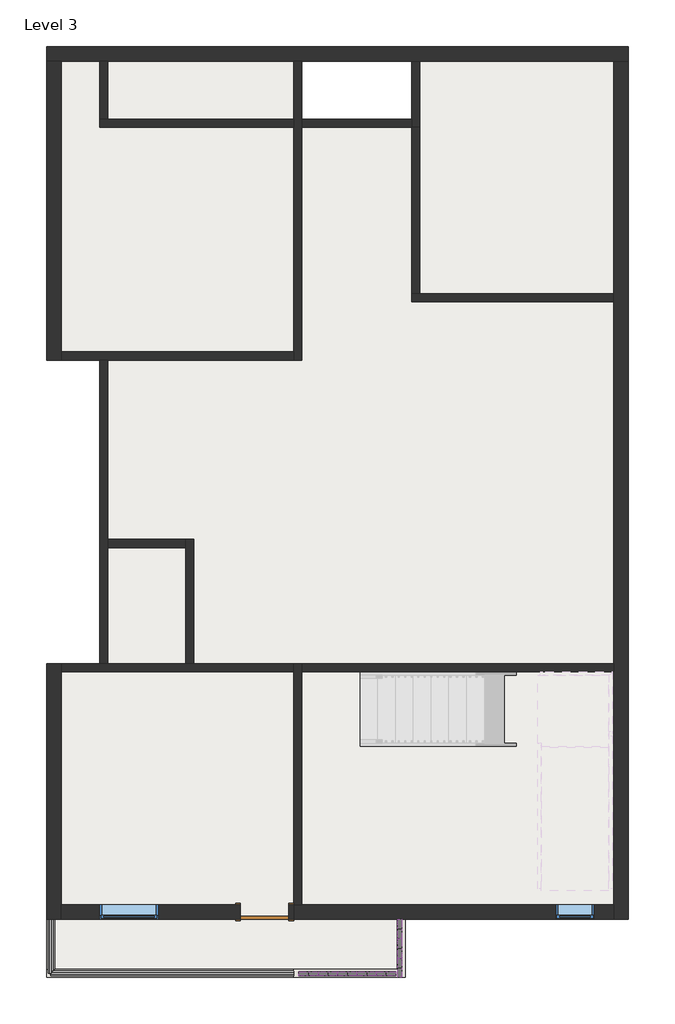
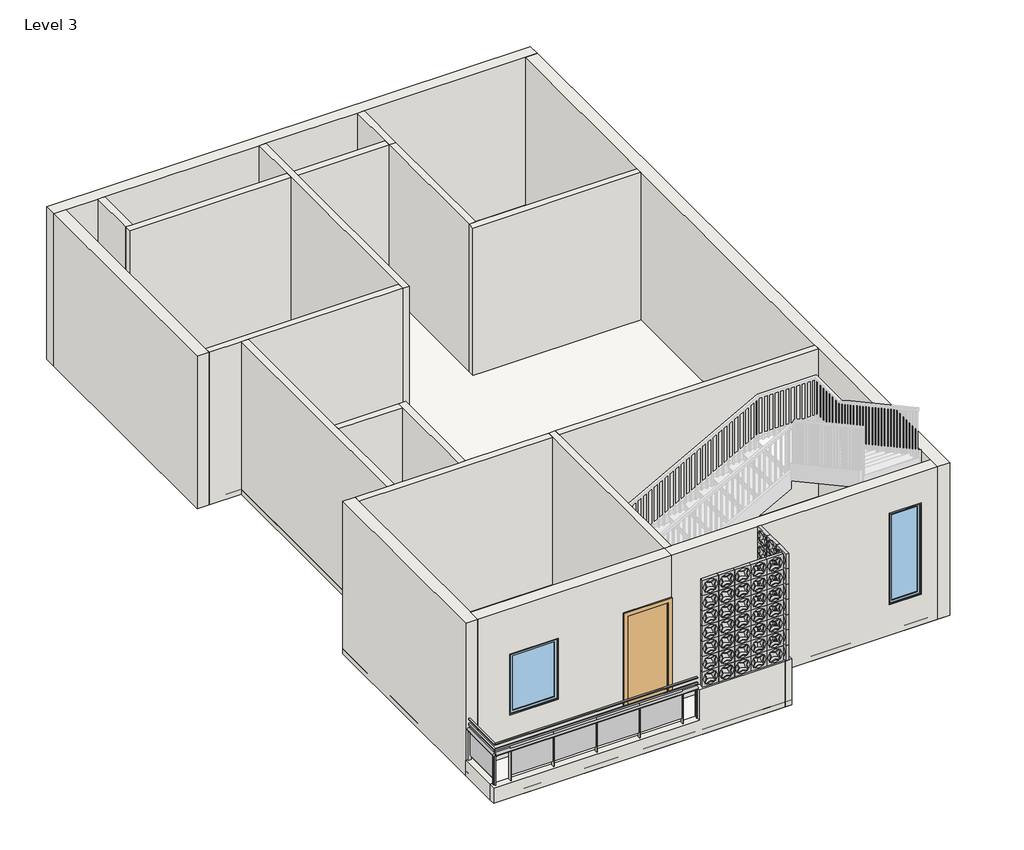
# One storey, part 1 of 2: 56 plates, 23 walls, 2 railings, 2 windows, 1 door, 1 roof.
"""IFC4 building model written with IfcOpenShell, lengths in millimetres."""

from ifc_helpers import new_model, si_unit, point, frame, origin, place, context, project, spatial, polyline, ellipse_curve, trimmed, outline, extrude, faceted_brep, transform, mapped, element, save
from ifc_brep_helpers import plane_surface, extruded_surface, advanced_brep
from components import door_5e1232af, plate_14329628, window_fc882ab3, fixed_4x3_c1f32544

model = new_model("IFC4")

# Units and contexts
model_context = context("Model", 3, world=origin())
ifc_project = project(units=[si_unit("LENGTHUNIT", "METRE", prefix="MILLI")], contexts=[model_context])

# Site, building, storey
site = spatial("IfcSite", under=ifc_project)
building = spatial("IfcBuilding", under=site)
storey = spatial("IfcBuildingStorey", under=building, Name="Level 3", Elevation=6096.0)

# Door
placement = place(None, origin())
door_shape = door_5e1232af(model_context)
element("IfcDoor", 1, ObjectType="Single-Flush : 30\" x 84\"", at=placement, inside=storey, context=model_context, shape_type="MappedRepresentation", body=[
    mapped(door_shape, transform((-1957.86646, -4503.4834702, 6096.0), x_axis=(1.0, 0.0, 0.0), y_axis=(0.0, 1.0, 0.0), z_axis=(0.0, 0.0, 1.0))),
])

# Plates
plate_shape = plate_14329628(model_context)
element("IfcPlate", 2, at=placement, inside=storey, context=model_context, shape_type="MappedRepresentation", body=[
    mapped(plate_shape, transform((194.78354, -4770.1834704, 7010.4), x_axis=(0.0, -1.0, 0.0), y_axis=(1.0, 0.0, 0.0), z_axis=(0.0, 0.0, 1.0))),
])
element("IfcPlate", 3, at=placement, inside=storey, context=model_context, shape_type="MappedRepresentation", body=[
    mapped(plate_shape, transform((194.78354, -5074.9834705, 7010.4), x_axis=(0.0, -1.0, 0.0), y_axis=(1.0, 0.0, 0.0), z_axis=(0.0, 0.0, 1.0))),
])
element("IfcPlate", 4, at=placement, inside=storey, context=model_context, shape_type="MappedRepresentation", body=[
    mapped(plate_shape, transform((194.78354, -5379.7834704, 7010.4), x_axis=(0.0, -1.0, 0.0), y_axis=(1.0, 0.0, 0.0), z_axis=(0.0, 0.0, 1.0))),
])
element("IfcPlate", 5, at=placement, inside=storey, context=model_context, shape_type="MappedRepresentation", body=[
    mapped(plate_shape, transform((194.78354, -4770.1834704, 7315.2), x_axis=(0.0, -1.0, 0.0), y_axis=(1.0, 0.0, 0.0), z_axis=(0.0, 0.0, 1.0))),
])
element("IfcPlate", 6, at=placement, inside=storey, context=model_context, shape_type="MappedRepresentation", body=[
    mapped(plate_shape, transform((194.78354, -5074.9834705, 7315.2), x_axis=(0.0, -1.0, 0.0), y_axis=(1.0, 0.0, 0.0), z_axis=(0.0, 0.0, 1.0))),
])
element("IfcPlate", 7, at=placement, inside=storey, context=model_context, shape_type="MappedRepresentation", body=[
    mapped(plate_shape, transform((194.78354, -5379.7834704, 7315.2), x_axis=(0.0, -1.0, 0.0), y_axis=(1.0, 0.0, 0.0), z_axis=(0.0, 0.0, 1.0))),
])
element("IfcPlate", 8, at=placement, inside=storey, context=model_context, shape_type="MappedRepresentation", body=[
    mapped(plate_shape, transform((194.78354, -4770.1834704, 7620.0), x_axis=(0.0, -1.0, 0.0), y_axis=(1.0, 0.0, 0.0), z_axis=(0.0, 0.0, 1.0))),
])
element("IfcPlate", 9, at=placement, inside=storey, context=model_context, shape_type="MappedRepresentation", body=[
    mapped(plate_shape, transform((194.78354, -5074.9834705, 7620.0), x_axis=(0.0, -1.0, 0.0), y_axis=(1.0, 0.0, 0.0), z_axis=(0.0, 0.0, 1.0))),
])
element("IfcPlate", 10, at=placement, inside=storey, context=model_context, shape_type="MappedRepresentation", body=[
    mapped(plate_shape, transform((194.78354, -5379.7834704, 7620.0), x_axis=(0.0, -1.0, 0.0), y_axis=(1.0, 0.0, 0.0), z_axis=(0.0, 0.0, 1.0))),
])
element("IfcPlate", 11, at=placement, inside=storey, context=model_context, shape_type="MappedRepresentation", body=[
    mapped(plate_shape, transform((194.78354, -4770.1834704, 7924.8), x_axis=(0.0, -1.0, 0.0), y_axis=(1.0, 0.0, 0.0), z_axis=(0.0, 0.0, 1.0))),
])
element("IfcPlate", 12, at=placement, inside=storey, context=model_context, shape_type="MappedRepresentation", body=[
    mapped(plate_shape, transform((194.78354, -5074.9834705, 7924.8), x_axis=(0.0, -1.0, 0.0), y_axis=(1.0, 0.0, 0.0), z_axis=(0.0, 0.0, 1.0))),
])
element("IfcPlate", 13, at=placement, inside=storey, context=model_context, shape_type="MappedRepresentation", body=[
    mapped(plate_shape, transform((194.78354, -5379.7834704, 7924.8), x_axis=(0.0, -1.0, 0.0), y_axis=(1.0, 0.0, 0.0), z_axis=(0.0, 0.0, 1.0))),
])
element("IfcPlate", 14, at=placement, inside=storey, context=model_context, shape_type="MappedRepresentation", body=[
    mapped(plate_shape, transform((194.78354, -4770.1834704, 8229.6), x_axis=(0.0, -1.0, 0.0), y_axis=(1.0, 0.0, 0.0), z_axis=(0.0, 0.0, 1.0))),
])
element("IfcPlate", 15, at=placement, inside=storey, context=model_context, shape_type="MappedRepresentation", body=[
    mapped(plate_shape, transform((194.78354, -5074.9834705, 8229.6), x_axis=(0.0, -1.0, 0.0), y_axis=(1.0, 0.0, 0.0), z_axis=(0.0, 0.0, 1.0))),
])
element("IfcPlate", 16, at=placement, inside=storey, context=model_context, shape_type="MappedRepresentation", body=[
    mapped(plate_shape, transform((194.78354, -5379.7834704, 8229.6), x_axis=(0.0, -1.0, 0.0), y_axis=(1.0, 0.0, 0.0), z_axis=(0.0, 0.0, 1.0))),
])
element("IfcPlate", 17, at=placement, inside=storey, context=model_context, shape_type="MappedRepresentation", body=[
    mapped(plate_shape, transform((194.78354, -4770.1834704, 8534.4), x_axis=(0.0, -1.0, 0.0), y_axis=(1.0, 0.0, 0.0), z_axis=(0.0, 0.0, 1.0))),
])
element("IfcPlate", 18, at=placement, inside=storey, context=model_context, shape_type="MappedRepresentation", body=[
    mapped(plate_shape, transform((194.78354, -5074.9834705, 8534.4), x_axis=(0.0, -1.0, 0.0), y_axis=(1.0, 0.0, 0.0), z_axis=(0.0, 0.0, 1.0))),
])
element("IfcPlate", 19, at=placement, inside=storey, context=model_context, shape_type="MappedRepresentation", body=[
    mapped(plate_shape, transform((194.78354, -5379.7834704, 8534.4), x_axis=(0.0, -1.0, 0.0), y_axis=(1.0, 0.0, 0.0), z_axis=(0.0, 0.0, 1.0))),
])
element("IfcPlate", 20, at=placement, inside=storey, context=model_context, shape_type="MappedRepresentation", body=[
    mapped(plate_shape, transform((194.78354, -4770.1834704, 8839.2), x_axis=(0.0, -1.0, 0.0), y_axis=(1.0, 0.0, 0.0), z_axis=(0.0, 0.0, 1.0))),
])
element("IfcPlate", 21, at=placement, inside=storey, context=model_context, shape_type="MappedRepresentation", body=[
    mapped(plate_shape, transform((194.78354, -5074.9834705, 8839.2), x_axis=(0.0, -1.0, 0.0), y_axis=(1.0, 0.0, 0.0), z_axis=(0.0, 0.0, 1.0))),
])
element("IfcPlate", 22, at=placement, inside=storey, context=model_context, shape_type="MappedRepresentation", body=[
    mapped(plate_shape, transform((194.78354, -5379.7834704, 8839.2), x_axis=(0.0, -1.0, 0.0), y_axis=(1.0, 0.0, 0.0), z_axis=(0.0, 0.0, 1.0))),
])
element("IfcPlate", 23, at=placement, inside=storey, context=model_context, shape_type="MappedRepresentation", body=[
    mapped(plate_shape, transform((-1272.0664598, -5443.2834702, 7010.4), x_axis=(1.0, 0.0, 0.0), y_axis=(0.0, 1.0, 0.0), z_axis=(0.0, 0.0, 1.0))),
])
element("IfcPlate", 24, at=placement, inside=storey, context=model_context, shape_type="MappedRepresentation", body=[
    mapped(plate_shape, transform((-967.2664597, -5443.2834702, 7010.4), x_axis=(1.0, 0.0, 0.0), y_axis=(0.0, 1.0, 0.0), z_axis=(0.0, 0.0, 1.0))),
])
element("IfcPlate", 25, at=placement, inside=storey, context=model_context, shape_type="MappedRepresentation", body=[
    mapped(plate_shape, transform((-662.4664597, -5443.2834702, 7010.4), x_axis=(1.0, 0.0, 0.0), y_axis=(0.0, 1.0, 0.0), z_axis=(0.0, 0.0, 1.0))),
])
element("IfcPlate", 26, at=placement, inside=storey, context=model_context, shape_type="MappedRepresentation", body=[
    mapped(plate_shape, transform((-1272.0664598, -5443.2834702, 7315.2), x_axis=(1.0, 0.0, 0.0), y_axis=(0.0, 1.0, 0.0), z_axis=(0.0, 0.0, 1.0))),
])
element("IfcPlate", 27, at=placement, inside=storey, context=model_context, shape_type="MappedRepresentation", body=[
    mapped(plate_shape, transform((-967.2664597, -5443.2834702, 7315.2), x_axis=(1.0, 0.0, 0.0), y_axis=(0.0, 1.0, 0.0), z_axis=(0.0, 0.0, 1.0))),
])
element("IfcPlate", 28, at=placement, inside=storey, context=model_context, shape_type="MappedRepresentation", body=[
    mapped(plate_shape, transform((-662.4664597, -5443.2834702, 7315.2), x_axis=(1.0, 0.0, 0.0), y_axis=(0.0, 1.0, 0.0), z_axis=(0.0, 0.0, 1.0))),
])
element("IfcPlate", 29, at=placement, inside=storey, context=model_context, shape_type="MappedRepresentation", body=[
    mapped(plate_shape, transform((-1272.0664598, -5443.2834702, 7620.0), x_axis=(1.0, 0.0, 0.0), y_axis=(0.0, 1.0, 0.0), z_axis=(0.0, 0.0, 1.0))),
])
element("IfcPlate", 30, at=placement, inside=storey, context=model_context, shape_type="MappedRepresentation", body=[
    mapped(plate_shape, transform((-967.2664597, -5443.2834702, 7620.0), x_axis=(1.0, 0.0, 0.0), y_axis=(0.0, 1.0, 0.0), z_axis=(0.0, 0.0, 1.0))),
])
element("IfcPlate", 31, at=placement, inside=storey, context=model_context, shape_type="MappedRepresentation", body=[
    mapped(plate_shape, transform((-662.4664597, -5443.2834702, 7620.0), x_axis=(1.0, 0.0, 0.0), y_axis=(0.0, 1.0, 0.0), z_axis=(0.0, 0.0, 1.0))),
])
element("IfcPlate", 32, at=placement, inside=storey, context=model_context, shape_type="MappedRepresentation", body=[
    mapped(plate_shape, transform((-1272.0664598, -5443.2834702, 7924.8), x_axis=(1.0, 0.0, 0.0), y_axis=(0.0, 1.0, 0.0), z_axis=(0.0, 0.0, 1.0))),
])
element("IfcPlate", 33, at=placement, inside=storey, context=model_context, shape_type="MappedRepresentation", body=[
    mapped(plate_shape, transform((-967.2664597, -5443.2834702, 7924.8), x_axis=(1.0, 0.0, 0.0), y_axis=(0.0, 1.0, 0.0), z_axis=(0.0, 0.0, 1.0))),
])
element("IfcPlate", 34, at=placement, inside=storey, context=model_context, shape_type="MappedRepresentation", body=[
    mapped(plate_shape, transform((-662.4664597, -5443.2834702, 7924.8), x_axis=(1.0, 0.0, 0.0), y_axis=(0.0, 1.0, 0.0), z_axis=(0.0, 0.0, 1.0))),
])
element("IfcPlate", 35, at=placement, inside=storey, context=model_context, shape_type="MappedRepresentation", body=[
    mapped(plate_shape, transform((-1272.0664598, -5443.2834702, 8229.6), x_axis=(1.0, 0.0, 0.0), y_axis=(0.0, 1.0, 0.0), z_axis=(0.0, 0.0, 1.0))),
])
element("IfcPlate", 36, at=placement, inside=storey, context=model_context, shape_type="MappedRepresentation", body=[
    mapped(plate_shape, transform((-967.2664597, -5443.2834702, 8229.6), x_axis=(1.0, 0.0, 0.0), y_axis=(0.0, 1.0, 0.0), z_axis=(0.0, 0.0, 1.0))),
])
element("IfcPlate", 37, at=placement, inside=storey, context=model_context, shape_type="MappedRepresentation", body=[
    mapped(plate_shape, transform((-662.4664597, -5443.2834702, 8229.6), x_axis=(1.0, 0.0, 0.0), y_axis=(0.0, 1.0, 0.0), z_axis=(0.0, 0.0, 1.0))),
])
element("IfcPlate", 38, at=placement, inside=storey, context=model_context, shape_type="MappedRepresentation", body=[
    mapped(plate_shape, transform((-1272.0664598, -5443.2834702, 8534.4), x_axis=(1.0, 0.0, 0.0), y_axis=(0.0, 1.0, 0.0), z_axis=(0.0, 0.0, 1.0))),
])
element("IfcPlate", 39, at=placement, inside=storey, context=model_context, shape_type="MappedRepresentation", body=[
    mapped(plate_shape, transform((-967.2664597, -5443.2834702, 8534.4), x_axis=(1.0, 0.0, 0.0), y_axis=(0.0, 1.0, 0.0), z_axis=(0.0, 0.0, 1.0))),
])
element("IfcPlate", 40, at=placement, inside=storey, context=model_context, shape_type="MappedRepresentation", body=[
    mapped(plate_shape, transform((-662.4664597, -5443.2834702, 8534.4), x_axis=(1.0, 0.0, 0.0), y_axis=(0.0, 1.0, 0.0), z_axis=(0.0, 0.0, 1.0))),
])
element("IfcPlate", 41, at=placement, inside=storey, context=model_context, shape_type="MappedRepresentation", body=[
    mapped(plate_shape, transform((-1272.0664598, -5443.2834702, 8839.2), x_axis=(1.0, 0.0, 0.0), y_axis=(0.0, 1.0, 0.0), z_axis=(0.0, 0.0, 1.0))),
])
element("IfcPlate", 42, at=placement, inside=storey, context=model_context, shape_type="MappedRepresentation", body=[
    mapped(plate_shape, transform((-967.2664597, -5443.2834702, 8839.2), x_axis=(1.0, 0.0, 0.0), y_axis=(0.0, 1.0, 0.0), z_axis=(0.0, 0.0, 1.0))),
])
element("IfcPlate", 43, at=placement, inside=storey, context=model_context, shape_type="MappedRepresentation", body=[
    mapped(plate_shape, transform((-662.4664597, -5443.2834702, 8839.2), x_axis=(1.0, 0.0, 0.0), y_axis=(0.0, 1.0, 0.0), z_axis=(0.0, 0.0, 1.0))),
])
element("IfcPlate", 44, at=placement, inside=storey, context=model_context, shape_type="MappedRepresentation", body=[
    mapped(plate_shape, transform((-357.6664597, -5443.2834702, 7010.4), x_axis=(1.0, 0.0, 0.0), y_axis=(0.0, 1.0, 0.0), z_axis=(0.0, 0.0, 1.0))),
])
element("IfcPlate", 45, at=placement, inside=storey, context=model_context, shape_type="MappedRepresentation", body=[
    mapped(plate_shape, transform((-357.6664597, -5443.2834702, 7315.2), x_axis=(1.0, 0.0, 0.0), y_axis=(0.0, 1.0, 0.0), z_axis=(0.0, 0.0, 1.0))),
])
element("IfcPlate", 46, at=placement, inside=storey, context=model_context, shape_type="MappedRepresentation", body=[
    mapped(plate_shape, transform((-357.6664597, -5443.2834702, 7620.0), x_axis=(1.0, 0.0, 0.0), y_axis=(0.0, 1.0, 0.0), z_axis=(0.0, 0.0, 1.0))),
])
element("IfcPlate", 47, at=placement, inside=storey, context=model_context, shape_type="MappedRepresentation", body=[
    mapped(plate_shape, transform((-357.6664597, -5443.2834702, 7924.8), x_axis=(1.0, 0.0, 0.0), y_axis=(0.0, 1.0, 0.0), z_axis=(0.0, 0.0, 1.0))),
])
element("IfcPlate", 48, at=placement, inside=storey, context=model_context, shape_type="MappedRepresentation", body=[
    mapped(plate_shape, transform((-357.6664597, -5443.2834702, 8229.6), x_axis=(1.0, 0.0, 0.0), y_axis=(0.0, 1.0, 0.0), z_axis=(0.0, 0.0, 1.0))),
])
element("IfcPlate", 49, at=placement, inside=storey, context=model_context, shape_type="MappedRepresentation", body=[
    mapped(plate_shape, transform((-357.6664597, -5443.2834702, 8534.4), x_axis=(1.0, 0.0, 0.0), y_axis=(0.0, 1.0, 0.0), z_axis=(0.0, 0.0, 1.0))),
])
element("IfcPlate", 50, at=placement, inside=storey, context=model_context, shape_type="MappedRepresentation", body=[
    mapped(plate_shape, transform((-357.6664597, -5443.2834702, 8839.2), x_axis=(1.0, 0.0, 0.0), y_axis=(0.0, 1.0, 0.0), z_axis=(0.0, 0.0, 1.0))),
])
element("IfcPlate", 51, at=placement, inside=storey, context=model_context, shape_type="MappedRepresentation", body=[
    mapped(plate_shape, transform((-52.8664598, -5443.2834702, 8839.2), x_axis=(1.0, 0.0, 0.0), y_axis=(0.0, 1.0, 0.0), z_axis=(0.0, 0.0, 1.0))),
])
element("IfcPlate", 52, at=placement, inside=storey, context=model_context, shape_type="MappedRepresentation", body=[
    mapped(plate_shape, transform((-52.8664598, -5443.2834702, 7010.4), x_axis=(1.0, 0.0, 0.0), y_axis=(0.0, 1.0, 0.0), z_axis=(0.0, 0.0, 1.0))),
])
element("IfcPlate", 53, at=placement, inside=storey, context=model_context, shape_type="MappedRepresentation", body=[
    mapped(plate_shape, transform((-52.8664598, -5443.2834702, 7315.2), x_axis=(1.0, 0.0, 0.0), y_axis=(0.0, 1.0, 0.0), z_axis=(0.0, 0.0, 1.0))),
])
element("IfcPlate", 54, at=placement, inside=storey, context=model_context, shape_type="MappedRepresentation", body=[
    mapped(plate_shape, transform((-52.8664598, -5443.2834702, 7620.0), x_axis=(1.0, 0.0, 0.0), y_axis=(0.0, 1.0, 0.0), z_axis=(0.0, 0.0, 1.0))),
])
element("IfcPlate", 55, at=placement, inside=storey, context=model_context, shape_type="MappedRepresentation", body=[
    mapped(plate_shape, transform((-52.8664598, -5443.2834702, 7924.8), x_axis=(1.0, 0.0, 0.0), y_axis=(0.0, 1.0, 0.0), z_axis=(0.0, 0.0, 1.0))),
])
element("IfcPlate", 56, at=placement, inside=storey, context=model_context, shape_type="MappedRepresentation", body=[
    mapped(plate_shape, transform((-52.8664598, -5443.2834702, 8229.6), x_axis=(1.0, 0.0, 0.0), y_axis=(0.0, 1.0, 0.0), z_axis=(0.0, 0.0, 1.0))),
])
element("IfcPlate", 57, at=placement, inside=storey, context=model_context, shape_type="MappedRepresentation", body=[
    mapped(plate_shape, transform((-52.8664598, -5443.2834702, 8534.4), x_axis=(1.0, 0.0, 0.0), y_axis=(0.0, 1.0, 0.0), z_axis=(0.0, 0.0, 1.0))),
])

# Railings
element("IfcRailing", 58, ObjectType="Glass Panel - Bottom Fill", at=placement, inside=storey, context=model_context, shape_type="SolidModel", body=[
    advanced_brep(
    [(-5285.26646, -4617.7834702, 7010.4), (-5361.46646, -4617.7834702, 7010.4), (-5285.26646, -5468.6834702, 7010.4), (-5361.46646, -5468.6834702, 7010.4)],
    [
        (0, 1, ellipse_curve(frame((-5323.36646, -4617.7834702, 7010.4), z_axis=(0.0, 1.0, 0.0), x_axis=(-1.0, 0.0, 0.0)), 38.1, 28.575)),
        (1, 0, ellipse_curve(frame((-5323.36646, -4617.7834702, 7010.4), z_axis=(0.0, 1.0, 0.0), x_axis=(-1.0, 0.0, 0.0)), 38.1, 28.575)),
        (2, 3, ellipse_curve(frame((-5323.36646, -5468.6834702, 7010.4), z_axis=(0.0, -1.0, 0.0), x_axis=(-1.0, 0.0, 0.0)), 38.1, 28.575)),
        (3, 2, ellipse_curve(frame((-5323.36646, -5468.6834702, 7010.4), z_axis=(0.0, -1.0, 0.0), x_axis=(-1.0, 0.0, 0.0)), 38.1, 28.575)),
        (0, 2),
        (3, 1),
    ],
    [
        plane_surface(frame((-5323.36646, -4617.7834702, 7010.4), z_axis=(0.0, 1.0, 0.0), x_axis=(0.0, 0.0, -1.0))),
        plane_surface(frame((-5323.36646, -5468.6834702, 7010.4), z_axis=(0.0, -1.0, 0.0), x_axis=(0.0, 0.0, -1.0))),
        extruded_surface(trimmed(ellipse_curve(frame((-5323.36646, -5468.6834702, 7010.4), z_axis=(0.0, 1.0, 0.0), x_axis=(-1.0, 0.0, 0.0)), 38.1, 28.575), [point((-5285.26646, -5468.6834702, 7010.4))], [point((-5361.46646, -5468.6834702, 7010.4))], True, "CARTESIAN"), (0.0, 850.8999999999996, 0.0), 850.8999999999996),
        extruded_surface(trimmed(ellipse_curve(frame((-5323.36646, -5468.6834702, 7010.4), z_axis=(0.0, 1.0, 0.0), x_axis=(-1.0, 0.0, 0.0)), 38.1, 28.575), [point((-5361.46646, -5468.6834702, 7010.4))], [point((-5285.26646, -5468.6834702, 7010.4))], True, "CARTESIAN"), (0.0, 850.8999999999996, 0.0), 850.8999999999996),
    ],
    [
        (0, [[1, 2]]),
        (1, [[3, 4]]),
        (2, [[-1, 5, -4, 6]]),
        (3, [[-2, -6, -3, -5]]),
    ],
),
    extrude(outline(polyline([(-5336.06646, -4617.7834702), (-5310.66646, -4617.7834702), (-5310.66646, -5468.6834702), (-5336.06646, -5468.6834702), (-5336.06646, -4617.7834702)])), frame((0.0, 0.0, 7200.9), z_axis=(0.0, 0.0, 1.0), x_axis=(1.0, 0.0, 0.0)), (0.0, 0.0, 1.0), 25.4),
    extrude(outline(polyline([(-5336.06646, -4617.7834702), (-5310.66646, -4617.7834702), (-5310.66646, -5468.6834702), (-5336.06646, -5468.6834702), (-5336.06646, -4617.7834702)])), frame((0.0, 0.0, 7099.3), z_axis=(0.0, 0.0, 1.0), x_axis=(1.0, 0.0, 0.0)), (0.0, 0.0, 1.0), 25.4),
    extrude(outline(polyline([(-5348.76646, -5443.2834702), (-5297.96646, -5443.2834702), (-5297.96646, -5455.9834702), (-5348.76646, -5455.9834702), (-5348.76646, -5443.2834702)])), frame((0.0, 0.0, 6400.8), z_axis=(0.0, 0.0, 1.0), x_axis=(1.0, 0.0, 0.0)), (0.0, 0.0, 1.0), 581.025),
    extrude(outline(polyline([(-5316.831303, -4636.8334702), (-5316.831303, -5449.6334702), (-5323.181303, -5449.6334702), (-5323.181303, -4636.8334702), (-5316.831303, -4636.8334702)])), frame((0.0, 0.0, 6502.4), z_axis=(0.0, 0.0, 1.0), x_axis=(1.0, 0.0, 0.0)), (0.0, 0.0, 1.0), 596.9),
    extrude(outline(polyline([(-5348.76646, -4630.4834702), (-5297.96646, -4630.4834702), (-5297.96646, -4643.1834702), (-5348.76646, -4643.1834702), (-5348.76646, -4630.4834702)])), frame((0.0, 0.0, 6400.8), z_axis=(0.0, 0.0, 1.0), x_axis=(1.0, 0.0, 0.0)), (0.0, 0.0, 1.0), 581.025),
    extrude(outline(polyline([(-5332.89146, -5455.9834702), (-5313.84146, -5455.9834702), (-5313.84146, -5475.0334702), (-5332.89146, -5475.0334702), (-5332.89146, -5455.9834702)])), frame((0.0, 0.0, 6400.8), z_axis=(0.0, 0.0, 1.0), x_axis=(1.0, 0.0, 0.0)), (0.0, 0.0, 1.0), 581.025),
    extrude(outline(polyline([(-5332.89146, -4611.4334702), (-5313.84146, -4611.4334702), (-5313.84146, -4630.4834702), (-5332.89146, -4630.4834702), (-5332.89146, -4611.4334702)])), frame((0.0, 0.0, 6400.8), z_axis=(0.0, 0.0, 1.0), x_axis=(1.0, 0.0, 0.0)), (0.0, 0.0, 1.0), 581.025),
])
element("IfcRailing", 59, ObjectType="Glass Panel - Bottom Fill", at=placement, inside=storey, context=model_context, shape_type="SolidModel", body=[
    advanced_brep(
    [(-1500.66646, -5506.7834702, 7010.4), (-1500.66646, -5430.5834702, 7010.4), (-5323.36646, -5506.7834702, 7010.4), (-5323.36646, -5430.5834702, 7010.4)],
    [
        (0, 1, ellipse_curve(frame((-1500.66646, -5468.6834702, 7010.4), z_axis=(1.0, 0.0, 0.0), x_axis=(0.0, 1.0, 0.0)), 38.1, 28.575)),
        (1, 0, ellipse_curve(frame((-1500.66646, -5468.6834702, 7010.4), z_axis=(1.0, 0.0, 0.0), x_axis=(0.0, 1.0, 0.0)), 38.1, 28.575)),
        (2, 3, ellipse_curve(frame((-5323.36646, -5468.6834702, 7010.4), z_axis=(-1.0, 0.0, 0.0), x_axis=(0.0, 1.0, 0.0)), 38.1, 28.575)),
        (3, 2, ellipse_curve(frame((-5323.36646, -5468.6834702, 7010.4), z_axis=(-1.0, 0.0, 0.0), x_axis=(0.0, 1.0, 0.0)), 38.1, 28.575)),
        (0, 2),
        (3, 1),
    ],
    [
        plane_surface(frame((-1500.66646, -5468.6834702, 7010.4), z_axis=(1.0, 0.0, 0.0), x_axis=(0.0, -1.0, 0.0))),
        plane_surface(frame((-5323.36646, -5468.6834702, 7010.4), z_axis=(-1.0, 0.0, 0.0), x_axis=(0.0, -1.0, 0.0))),
        extruded_surface(trimmed(ellipse_curve(frame((-5323.36646, -5468.6834702, 7010.4), z_axis=(1.0, 0.0, 0.0), x_axis=(0.0, 1.0, 0.0)), 38.1, 28.575), [point((-5323.36646, -5506.7834702, 7010.4))], [point((-5323.36646, -5430.5834702, 7010.4))], True, "CARTESIAN"), (3822.7000000000003, 0.0, 0.0), 3822.7000000000003),
        extruded_surface(trimmed(ellipse_curve(frame((-5323.36646, -5468.6834702, 7010.4), z_axis=(1.0, 0.0, 0.0), x_axis=(0.0, 1.0, 0.0)), 38.1, 28.575), [point((-5323.36646, -5430.5834702, 7010.4))], [point((-5323.36646, -5506.7834702, 7010.4))], True, "CARTESIAN"), (3822.7000000000003, 0.0, 0.0), 3822.7000000000003),
    ],
    [
        (0, [[1, 2]]),
        (1, [[3, 4]]),
        (2, [[-1, 5, -4, 6]]),
        (3, [[-2, -6, -3, -5]]),
    ],
),
    extrude(outline(polyline([(-1500.66646, -5455.9834702), (-1500.66646, -5481.3834702), (-5323.36646, -5481.3834702), (-5323.36646, -5455.9834702), (-1500.66646, -5455.9834702)])), frame((0.0, 0.0, 7200.9), z_axis=(0.0, 0.0, 1.0), x_axis=(1.0, 0.0, 0.0)), (0.0, 0.0, 1.0), 25.4),
    extrude(outline(polyline([(-1500.66646, -5455.9834702), (-1500.66646, -5481.3834702), (-5323.36646, -5481.3834702), (-5323.36646, -5455.9834702), (-1500.66646, -5455.9834702)])), frame((0.0, 0.0, 7099.3), z_axis=(0.0, 0.0, 1.0), x_axis=(1.0, 0.0, 0.0)), (0.0, 0.0, 1.0), 25.4),
    extrude(outline(polyline([(-5031.26646, -5443.2834702), (-5031.26646, -5494.0834702), (-5043.96646, -5494.0834702), (-5043.96646, -5443.2834702), (-5031.26646, -5443.2834702)])), frame((0.0, 0.0, 6400.8), z_axis=(0.0, 0.0, 1.0), x_axis=(1.0, 0.0, 0.0)), (0.0, 0.0, 1.0), 581.025),
    extrude(outline(polyline([(-4224.81646, -5475.2186272), (-5037.61646, -5475.2186272), (-5037.61646, -5468.8686272), (-4224.81646, -5468.8686272), (-4224.81646, -5475.2186272)])), frame((0.0, 0.0, 6502.4), z_axis=(0.0, 0.0, 1.0), x_axis=(1.0, 0.0, 0.0)), (0.0, 0.0, 1.0), 596.9),
    extrude(outline(polyline([(-4218.46646, -5443.2834702), (-4218.46646, -5494.0834702), (-4231.16646, -5494.0834702), (-4231.16646, -5443.2834702), (-4218.46646, -5443.2834702)])), frame((0.0, 0.0, 6400.8), z_axis=(0.0, 0.0, 1.0), x_axis=(1.0, 0.0, 0.0)), (0.0, 0.0, 1.0), 581.025),
    extrude(outline(polyline([(-3412.01646, -5475.2186272), (-4224.81646, -5475.2186272), (-4224.81646, -5468.8686272), (-3412.01646, -5468.8686272), (-3412.01646, -5475.2186272)])), frame((0.0, 0.0, 6502.4), z_axis=(0.0, 0.0, 1.0), x_axis=(1.0, 0.0, 0.0)), (0.0, 0.0, 1.0), 596.9),
    extrude(outline(polyline([(-3405.66646, -5443.2834702), (-3405.66646, -5494.0834702), (-3418.36646, -5494.0834702), (-3418.36646, -5443.2834702), (-3405.66646, -5443.2834702)])), frame((0.0, 0.0, 6400.8), z_axis=(0.0, 0.0, 1.0), x_axis=(1.0, 0.0, 0.0)), (0.0, 0.0, 1.0), 581.025),
    extrude(outline(polyline([(-2599.21646, -5475.2186272), (-3412.01646, -5475.2186272), (-3412.01646, -5468.8686272), (-2599.21646, -5468.8686272), (-2599.21646, -5475.2186272)])), frame((0.0, 0.0, 6502.4), z_axis=(0.0, 0.0, 1.0), x_axis=(1.0, 0.0, 0.0)), (0.0, 0.0, 1.0), 596.9),
    extrude(outline(polyline([(-2592.86646, -5443.2834702), (-2592.86646, -5494.0834702), (-2605.56646, -5494.0834702), (-2605.56646, -5443.2834702), (-2592.86646, -5443.2834702)])), frame((0.0, 0.0, 6400.8), z_axis=(0.0, 0.0, 1.0), x_axis=(1.0, 0.0, 0.0)), (0.0, 0.0, 1.0), 581.025),
    extrude(outline(polyline([(-1786.41646, -5475.2186272), (-2599.21646, -5475.2186272), (-2599.21646, -5468.8686272), (-1786.41646, -5468.8686272), (-1786.41646, -5475.2186272)])), frame((0.0, 0.0, 6502.4), z_axis=(0.0, 0.0, 1.0), x_axis=(1.0, 0.0, 0.0)), (0.0, 0.0, 1.0), 596.9),
    extrude(outline(polyline([(-1780.06646, -5443.2834702), (-1780.06646, -5494.0834702), (-1792.76646, -5494.0834702), (-1792.76646, -5443.2834702), (-1780.06646, -5443.2834702)])), frame((0.0, 0.0, 6400.8), z_axis=(0.0, 0.0, 1.0), x_axis=(1.0, 0.0, 0.0)), (0.0, 0.0, 1.0), 581.025),
    extrude(outline(polyline([(-5310.66646, -5459.1584702), (-5310.66646, -5478.2084702), (-5329.71646, -5478.2084702), (-5329.71646, -5459.1584702), (-5310.66646, -5459.1584702)])), frame((0.0, 0.0, 6400.8), z_axis=(0.0, 0.0, 1.0), x_axis=(1.0, 0.0, 0.0)), (0.0, 0.0, 1.0), 581.025),
    extrude(outline(polyline([(-1494.31646, -5459.1584702), (-1494.31646, -5478.2084702), (-1513.36646, -5478.2084702), (-1513.36646, -5459.1584702), (-1494.31646, -5459.1584702)])), frame((0.0, 0.0, 6400.8), z_axis=(0.0, 0.0, 1.0), x_axis=(1.0, 0.0, 0.0)), (0.0, 0.0, 1.0), 581.025),
])

# Roof
element("IfcRoof", 60, ObjectType="Generic - 4\"", at=placement, inside=storey, context=model_context, shape_type="Brep", body=[
    faceted_brep([(-5386.86646, 4170.6165298, 6096.0), (-5386.86646, 9098.2165298, 6096.0), (3757.13354, 9098.2165298, 6096.0), (3757.13354, -4617.7834702, 6096.0), (251.93354, -4617.7834702, 6096.0), (251.93354, -5532.1834702, 6096.0), (-5386.86646, -5532.1834702, 6096.0), (-5386.86646, -604.5834702, 6096.0), (-5158.26646, -604.5834702, 6096.0), (-4548.66646, -604.5834702, 6096.0), (-4548.66646, 4170.6165298, 6096.0), (-5158.26646, 4170.6165298, 6096.0), (353.53354, 8869.6165298, 6096.0), (-1373.66646, 8869.6165298, 6096.0), (-1373.66646, 7955.2165298, 6096.0), (353.53354, 7955.2165298, 6096.0), (3757.13354, -4617.7834702, 6197.6), (3757.13354, 9098.2165298, 6197.6), (-5386.86646, 9098.2165298, 6197.6), (-5386.86646, 4170.6165298, 6197.6), (-5158.26646, 4170.6165298, 6197.6), (-4548.66646, 4170.6165298, 6197.6), (-4548.66646, -604.5834702, 6197.6), (-5158.26646, -604.5834702, 6197.6), (-5386.86646, -604.5834702, 6197.6), (-5386.86646, -5532.1834702, 6197.6), (251.93354, -5532.1834702, 6197.6), (251.93354, -4617.7834702, 6197.6), (-1373.66646, 8869.6165298, 6197.6), (353.53354, 8869.6165298, 6197.6), (353.53354, 7955.2165298, 6197.6), (-1373.66646, 7955.2165298, 6197.6)], [[[0, 1, 2, 3, 4, 5, 6, 7, 8, 9, 10, 11], [12, 13, 14, 15]], [[16, 17, 18, 19, 20, 21, 22, 23, 24, 25, 26, 27], [28, 29, 30, 31]], [[2, 1, 18, 17]], [[1, 0, 19, 18]], [[3, 2, 17, 16]], [[4, 3, 16, 27]], [[5, 4, 27, 26]], [[6, 5, 26, 25]], [[22, 9, 8, 7, 24, 23]], [[10, 9, 22, 21]], [[19, 0, 11, 10, 21, 20]], [[7, 6, 25, 24]], [[12, 29, 28, 13]], [[13, 28, 31, 14]], [[14, 31, 30, 15]], [[29, 12, 15, 30]]]),
])

# Walls
element("IfcWall", 61, ObjectType="Generic - 5\"", at=placement, inside=storey, context=model_context, shape_type="Brep", body=[
    faceted_brep([(-1500.66646, -604.5834702, 6096.0), (-3075.46646, -604.5834702, 6096.0), (-3202.46646, -604.5834702, 6096.0), (-4421.66646, -604.5834702, 6096.0), (-4548.66646, -604.5834702, 6096.0), (-5158.26646, -604.5834702, 6096.0), (-5158.26646, -604.5834702, 9144.0), (-4548.66646, -604.5834702, 9144.0), (-4421.66646, -604.5834702, 9144.0), (-3202.46646, -604.5834702, 9144.0), (-3075.46646, -604.5834702, 9144.0), (-1500.66646, -604.5834702, 9144.0), (-1500.66646, -731.5834702, 6096.0), (-1500.66646, -731.5834702, 9144.0), (-5158.26646, -731.5834702, 9144.0), (-5158.26646, -731.5834702, 6096.0)], [[[0, 1, 2, 3, 4, 5, 6, 7, 8, 9, 10, 11]], [[12, 13, 14, 15]], [[5, 4, 3, 2, 1, 0, 12, 15]], [[11, 10, 9, 8, 7, 6, 14, 13]], [[0, 11, 13, 12]], [[6, 5, 15, 14]]]),
])
element("IfcWall", 62, ObjectType="Generic - 5\"", at=placement, inside=storey, context=model_context, shape_type="SweptSolid", body=[
    extrude(outline(polyline([(3528.53354, -731.5834702), (-1373.66646, -731.5834702), (-1373.66646, -604.5834702), (3528.53354, -604.5834702), (3528.53354, -731.5834702)])), frame((0.0, 0.0, 6096.0), z_axis=(0.0, 0.0, 1.0), x_axis=(1.0, 0.0, 0.0)), (0.0, 0.0, 1.0), 3048.0),
])
element("IfcWall", 63, ObjectType="Generic - 5\"", at=placement, inside=storey, context=model_context, shape_type="Brep", body=[
    faceted_brep([(-1500.66646, 8869.6165298, 6096.0), (-1500.66646, 7955.2165298, 6096.0), (-1500.66646, 7828.2165298, 6096.0), (-1500.66646, 4297.6165298, 6096.0), (-1500.66646, 4170.6165298, 6096.0), (-1500.66646, 4170.6165298, 9144.0), (-1500.66646, 4297.6165298, 9144.0), (-1500.66646, 7828.2165298, 9144.0), (-1500.66646, 7955.2165298, 9144.0), (-1500.66646, 8869.6165298, 9144.0), (-1373.66646, 8869.6165298, 6096.0), (-1373.66646, 8869.6165298, 9144.0), (-1373.66646, 7955.2165298, 9144.0), (-1373.66646, 7828.2165298, 9144.0), (-1373.66646, 4170.6165298, 9144.0), (-1373.66646, 4170.6165298, 6096.0), (-1373.66646, 7828.2165298, 6096.0), (-1373.66646, 7955.2165298, 6096.0)], [[[0, 1, 2, 3, 4, 5, 6, 7, 8, 9]], [[10, 11, 12, 13, 14, 15, 16, 17]], [[4, 3, 2, 1, 0, 10, 17, 16, 15]], [[9, 8, 7, 6, 5, 14, 13, 12, 11]], [[0, 9, 11, 10]], [[5, 4, 15, 14]]]),
])
element("IfcWall", 64, ObjectType="Generic - 5\"", at=placement, inside=storey, context=model_context, shape_type="Brep", body=[
    faceted_brep([(-1500.66646, 4297.6165298, 6096.0), (-5158.26646, 4297.6165298, 6096.0), (-5158.26646, 4297.6165298, 9144.0), (-1500.66646, 4297.6165298, 9144.0), (-1500.66646, 4170.6165298, 6096.0), (-1500.66646, 4170.6165298, 9144.0), (-4421.66646, 4170.6165298, 9144.0), (-4548.66646, 4170.6165298, 9144.0), (-5158.26646, 4170.6165298, 9144.0), (-5158.26646, 4170.6165298, 6096.0), (-4548.66646, 4170.6165298, 6096.0), (-4421.66646, 4170.6165298, 6096.0)], [[[0, 1, 2, 3]], [[4, 5, 6, 7, 8, 9, 10, 11]], [[1, 0, 4, 11, 10, 9]], [[3, 2, 8, 7, 6, 5]], [[0, 3, 5, 4]], [[2, 1, 9, 8]]]),
])
element("IfcWall", 65, ObjectType="Generic - 5\"", at=placement, inside=storey, context=model_context, shape_type="Brep", body=[
    faceted_brep([(353.53354, 8869.6165298, 6096.0), (353.53354, 7955.2165298, 6096.0), (353.53354, 7828.2165298, 6096.0), (353.53354, 7828.2165298, 9144.0), (353.53354, 7955.2165298, 9144.0), (353.53354, 8869.6165298, 9144.0), (480.53354, 8869.6165298, 6096.0), (480.53354, 8869.6165298, 9144.0), (480.53354, 7828.2165298, 9144.0), (480.53354, 7828.2165298, 6096.0)], [[[0, 1, 2, 3, 4, 5]], [[6, 7, 8, 9]], [[2, 1, 0, 6, 9]], [[5, 4, 3, 8, 7]], [[0, 5, 7, 6]], [[3, 2, 9, 8]]]),
])
element("IfcWall", 66, ObjectType="Generic - 5\"", at=placement, inside=storey, context=model_context, shape_type="SweptSolid", body=[
    extrude(outline(polyline([(-1373.66646, 7955.2165298), (353.53354, 7955.2165298), (353.53354, 7828.2165298), (-1373.66646, 7828.2165298), (-1373.66646, 7955.2165298)])), frame((0.0, 0.0, 6096.0), z_axis=(0.0, 0.0, 1.0), x_axis=(1.0, 0.0, 0.0)), (0.0, 0.0, 1.0), 3048.0),
])
element("IfcWall", 67, ObjectType="Generic - 5\"", at=placement, inside=storey, context=model_context, shape_type="Brep", body=[
    faceted_brep([(3528.53354, 5212.0165298, 6096.0), (480.53354, 5212.0165298, 6096.0), (353.53354, 5212.0165298, 6096.0), (353.53354, 5212.0165298, 9144.0), (480.53354, 5212.0165298, 9144.0), (3528.53354, 5212.0165298, 9144.0), (3528.53354, 5085.0165298, 6096.0), (3528.53354, 5085.0165298, 9144.0), (353.53354, 5085.0165298, 9144.0), (353.53354, 5085.0165298, 6096.0)], [[[0, 1, 2, 3, 4, 5]], [[6, 7, 8, 9]], [[2, 1, 0, 6, 9]], [[5, 4, 3, 8, 7]], [[0, 5, 7, 6]], [[3, 2, 9, 8]]]),
])
element("IfcWall", 68, ObjectType="Generic - 5\"", at=placement, inside=storey, context=model_context, shape_type="SweptSolid", body=[
    extrude(outline(polyline([(480.53354, 7828.2165298), (480.53354, 5212.0165298), (353.53354, 5212.0165298), (353.53354, 7828.2165298), (480.53354, 7828.2165298)])), frame((0.0, 0.0, 6096.0), z_axis=(0.0, 0.0, 1.0), x_axis=(1.0, 0.0, 0.0)), (0.0, 0.0, 1.0), 3048.0),
])
element("IfcWall", 69, ObjectType="Generic - 5\"", at=placement, inside=storey, context=model_context, shape_type="Brep", body=[
    faceted_brep([(-4421.66646, -604.5834702, 6096.0), (-4421.66646, 1224.2165298, 6096.0), (-4421.66646, 1351.2165298, 6096.0), (-4421.66646, 4170.6165298, 6096.0), (-4421.66646, 4170.6165298, 9144.0), (-4421.66646, 1351.2165298, 9144.0), (-4421.66646, 1224.2165298, 9144.0), (-4421.66646, -604.5834702, 9144.0), (-4548.66646, -604.5834702, 6096.0), (-4548.66646, -604.5834702, 9144.0), (-4548.66646, 4170.6165298, 9144.0), (-4548.66646, 4170.6165298, 6096.0)], [[[0, 1, 2, 3, 4, 5, 6, 7]], [[8, 9, 10, 11]], [[3, 2, 1, 0, 8, 11]], [[7, 6, 5, 4, 10, 9]], [[0, 7, 9, 8]], [[4, 3, 11, 10]]]),
])
element("IfcWall", 70, ObjectType="Generic - 5\"", at=placement, inside=storey, context=model_context, shape_type="Brep", body=[
    faceted_brep([(-3075.46646, -604.5834702, 6096.0), (-3075.46646, 1351.2165298, 6096.0), (-3075.46646, 1351.2165298, 9144.0), (-3075.46646, -604.5834702, 9144.0), (-3202.46646, -604.5834702, 6096.0), (-3202.46646, -604.5834702, 9144.0), (-3202.46646, 1224.2165298, 9144.0), (-3202.46646, 1351.2165298, 9144.0), (-3202.46646, 1351.2165298, 6096.0), (-3202.46646, 1224.2165298, 6096.0)], [[[0, 1, 2, 3]], [[4, 5, 6, 7, 8, 9]], [[1, 0, 4, 9, 8]], [[3, 2, 7, 6, 5]], [[0, 3, 5, 4]], [[2, 1, 8, 7]]]),
])
element("IfcWall", 71, ObjectType="Generic - 5\"", at=placement, inside=storey, context=model_context, shape_type="SweptSolid", body=[
    extrude(outline(polyline([(-4421.66646, 1351.2165298), (-3202.46646, 1351.2165298), (-3202.46646, 1224.2165298), (-4421.66646, 1224.2165298), (-4421.66646, 1351.2165298)])), frame((0.0, 0.0, 6096.0), z_axis=(0.0, 0.0, 1.0), x_axis=(1.0, 0.0, 0.0)), (0.0, 0.0, 1.0), 3048.0),
])
element("IfcWall", 72, ObjectType="Generic - 5\"", at=placement, inside=storey, context=model_context, shape_type="Brep", body=[
    faceted_brep([(-1500.66646, 7955.2165298, 6096.0), (-4421.66646, 7955.2165298, 6096.0), (-4548.66646, 7955.2165298, 6096.0), (-4548.66646, 7955.2165298, 9144.0), (-4421.66646, 7955.2165298, 9144.0), (-1500.66646, 7955.2165298, 9144.0), (-1500.66646, 7828.2165298, 6096.0), (-1500.66646, 7828.2165298, 9144.0), (-4548.66646, 7828.2165298, 9144.0), (-4548.66646, 7828.2165298, 6096.0)], [[[0, 1, 2, 3, 4, 5]], [[6, 7, 8, 9]], [[2, 1, 0, 6, 9]], [[5, 4, 3, 8, 7]], [[0, 5, 7, 6]], [[3, 2, 9, 8]]]),
])
element("IfcWall", 73, ObjectType="Generic - 5\"", at=placement, inside=storey, context=model_context, shape_type="SweptSolid", body=[
    extrude(outline(polyline([(-4421.66646, 8869.6165298), (-4421.66646, 7955.2165298), (-4548.66646, 7955.2165298), (-4548.66646, 8869.6165298), (-4421.66646, 8869.6165298)])), frame((0.0, 0.0, 6096.0), z_axis=(0.0, 0.0, 1.0), x_axis=(1.0, 0.0, 0.0)), (0.0, 0.0, 1.0), 3048.0),
])
element("IfcWall", 74, ObjectType="Generic - 5\"", at=placement, inside=storey, context=model_context, shape_type="Brep", body=[
    faceted_brep([(-1373.66646, -4389.1834702, 6096.0), (-1373.66646, -731.5834702, 6096.0), (-1373.66646, -604.5834702, 6096.0), (-1373.66646, -604.5834702, 9144.0), (-1373.66646, -731.5834702, 9144.0), (-1373.66646, -4389.1834702, 9144.0), (-1500.66646, -4389.1834702, 6096.0), (-1500.66646, -4389.1834702, 9144.0), (-1500.66646, -731.5834702, 9144.0), (-1500.66646, -604.5834702, 9144.0), (-1500.66646, -604.5834702, 6096.0), (-1500.66646, -731.5834702, 6096.0)], [[[0, 1, 2, 3, 4, 5]], [[6, 7, 8, 9, 10, 11]], [[2, 1, 0, 6, 11, 10]], [[5, 4, 3, 9, 8, 7]], [[3, 2, 10, 9]], [[0, 5, 7, 6]]]),
])
element("IfcWall", 75, ObjectType="Generic - 5\"", at=placement, inside=storey, context=model_context, shape_type="Brep", body=[
    faceted_brep([(124.93354, -4617.7834702, 6096.0), (124.93354, -5405.1834702, 6096.0), (124.93354, -5532.1834702, 6096.0), (124.93354, -5532.1834702, 7010.4), (124.93354, -5405.1834702, 7010.4), (124.93354, -4617.7834702, 7010.4), (251.93354, -4617.7834702, 6096.0), (251.93354, -4617.7834702, 7010.4), (251.93354, -5532.1834702, 7010.4), (251.93354, -5532.1834702, 6096.0)], [[[0, 1, 2, 3, 4, 5]], [[6, 7, 8, 9]], [[2, 1, 0, 6, 9]], [[5, 4, 3, 8, 7]], [[3, 2, 9, 8]], [[0, 5, 7, 6]]]),
])
element("IfcWall", 76, ObjectType="Generic - 5\"", at=placement, inside=storey, context=model_context, shape_type="Brep", body=[
    faceted_brep([(124.93354, -5405.1834702, 6096.0), (-5259.86646, -5405.1834702, 6096.0), (-5386.86646, -5405.1834702, 6096.0), (-5386.86646, -5405.1834702, 6400.8), (-5259.86646, -5405.1834702, 6400.8), (-1500.66646, -5405.1834702, 6400.8), (-1500.66646, -5405.1834702, 7010.4), (124.93354, -5405.1834702, 7010.4), (124.93354, -5532.1834702, 6096.0), (124.93354, -5532.1834702, 7010.4), (-1500.66646, -5532.1834702, 7010.4), (-1500.66646, -5532.1834702, 6400.8), (-5386.86646, -5532.1834702, 6400.8), (-5386.86646, -5532.1834702, 6096.0)], [[[0, 1, 2, 3, 4, 5, 6, 7]], [[8, 9, 10, 11, 12, 13]], [[0, 7, 9, 8]], [[3, 2, 13, 12]], [[2, 1, 0, 8, 13]], [[5, 4, 3, 12, 11]], [[6, 5, 11, 10]], [[7, 6, 10, 9]]]),
])
element("IfcWall", 77, ObjectType="Generic - 5\"", at=placement, inside=storey, context=model_context, shape_type="SweptSolid", body=[
    extrude(outline(polyline([(-5259.86646, -4617.7834702), (-5259.86646, -5405.1834702), (-5386.86646, -5405.1834702), (-5386.86646, -4617.7834702), (-5259.86646, -4617.7834702)])), frame((0.0, 0.0, 6096.0), z_axis=(0.0, 0.0, 1.0), x_axis=(1.0, 0.0, 0.0)), (0.0, 0.0, 1.0), 304.8),
])
element("IfcWall", 78, ObjectType="Generic -9\"", at=placement, inside=storey, context=model_context, shape_type="Brep", body=[
    faceted_brep([(-5386.86646, 8869.6165298, 6096.0), (-5158.26646, 8869.6165298, 6096.0), (-4548.66646, 8869.6165298, 6096.0), (-4421.66646, 8869.6165298, 6096.0), (-1500.66646, 8869.6165298, 6096.0), (-1373.66646, 8869.6165298, 6096.0), (353.53354, 8869.6165298, 6096.0), (480.53354, 8869.6165298, 6096.0), (3528.53354, 8869.6165298, 6096.0), (3757.13354, 8869.6165298, 6096.0), (3757.13354, 8869.6165298, 9144.0), (3528.53354, 8869.6165298, 9144.0), (480.53354, 8869.6165298, 9144.0), (353.53354, 8869.6165298, 9144.0), (-1373.66646, 8869.6165298, 9144.0), (-1500.66646, 8869.6165298, 9144.0), (-4421.66646, 8869.6165298, 9144.0), (-4548.66646, 8869.6165298, 9144.0), (-5158.26646, 8869.6165298, 9144.0), (-5386.86646, 8869.6165298, 9144.0), (-5386.86646, 9098.2165298, 6096.0), (-5386.86646, 9098.2165298, 9144.0), (3757.13354, 9098.2165298, 9144.0), (3757.13354, 9098.2165298, 6096.0)], [[[0, 1, 2, 3, 4, 5, 6, 7, 8, 9, 10, 11, 12, 13, 14, 15, 16, 17, 18, 19]], [[20, 21, 22, 23]], [[9, 8, 7, 6, 5, 4, 3, 2, 1, 0, 20, 23]], [[19, 18, 17, 16, 15, 14, 13, 12, 11, 10, 22, 21]], [[10, 9, 23, 22]], [[0, 19, 21, 20]]]),
])
element("IfcWall", 79, ObjectType="Generic -9\"", at=placement, inside=storey, context=model_context, shape_type="Brep", body=[
    faceted_brep([(3528.53354, 8869.6165298, 6096.0), (3528.53354, 5212.0165298, 6096.0), (3528.53354, 5085.0165298, 6096.0), (3528.53354, -604.5834702, 6096.0), (3528.53354, -731.5834702, 6096.0), (3528.53354, -4389.1834702, 6096.0), (3528.53354, -4617.7834702, 6096.0), (3528.53354, -4617.7834702, 9144.0), (3528.53354, -4389.1834702, 9144.0), (3528.53354, -731.5834702, 9144.0), (3528.53354, -604.5834702, 9144.0), (3528.53354, 5085.0165298, 9144.0), (3528.53354, 5212.0165298, 9144.0), (3528.53354, 8869.6165298, 9144.0), (3757.13354, 8869.6165298, 6096.0), (3757.13354, 8869.6165298, 9144.0), (3757.13354, -4617.7834702, 9144.0), (3757.13354, -4617.7834702, 6096.0)], [[[0, 1, 2, 3, 4, 5, 6, 7, 8, 9, 10, 11, 12, 13]], [[14, 15, 16, 17]], [[6, 5, 4, 3, 2, 1, 0, 14, 17]], [[13, 12, 11, 10, 9, 8, 7, 16, 15]], [[0, 13, 15, 14]], [[7, 6, 17, 16]]]),
])
element("IfcWall", 80, ObjectType="Generic -9\"", at=placement, inside=storey, context=model_context, shape_type="Brep", body=[
    faceted_brep([(3528.53354, -4389.1834702, 6096.0), (-1373.66646, -4389.1834702, 6096.0), (-1500.66646, -4389.1834702, 6096.0), (-1500.66646, -4389.1834702, 9144.0), (-1373.66646, -4389.1834702, 9144.0), (3528.53354, -4389.1834702, 9144.0), (2614.13354, -4389.1834702, 8534.4), (2614.13354, -4389.1834702, 6705.6), (3223.73354, -4389.1834702, 6705.6), (3223.73354, -4389.1834702, 8534.4), (3528.53354, -4617.7834702, 6096.0), (3528.53354, -4617.7834702, 9144.0), (-1500.66646, -4617.7834702, 9144.0), (-1500.66646, -4617.7834702, 6096.0), (124.93354, -4617.7834702, 6096.0), (251.93354, -4617.7834702, 6096.0), (2614.13354, -4617.7834702, 8534.4), (3223.73354, -4617.7834702, 8534.4), (3223.73354, -4617.7834702, 6705.6), (2614.13354, -4617.7834702, 6705.6)], [[[0, 1, 2, 3, 4, 5], [6, 7, 8, 9]], [[10, 11, 12, 13, 14, 15], [16, 17, 18, 19]], [[2, 1, 0, 10, 15, 14, 13]], [[5, 4, 3, 12, 11]], [[0, 5, 11, 10]], [[7, 6, 16, 19]], [[8, 7, 19, 18]], [[9, 8, 18, 17]], [[6, 9, 17, 16]], [[3, 2, 13, 12]]]),
])
element("IfcWall", 81, ObjectType="Generic -9\"", at=placement, inside=storey, context=model_context, shape_type="Brep", body=[
    faceted_brep([(-5158.26646, 4170.6165298, 6096.0), (-5158.26646, 4297.6165298, 6096.0), (-5158.26646, 8869.6165298, 6096.0), (-5158.26646, 8869.6165298, 9144.0), (-5158.26646, 4297.6165298, 9144.0), (-5158.26646, 4170.6165298, 9144.0), (-5386.86646, 4170.6165298, 6096.0), (-5386.86646, 4170.6165298, 9144.0), (-5386.86646, 8869.6165298, 9144.0), (-5386.86646, 8869.6165298, 6096.0)], [[[0, 1, 2, 3, 4, 5]], [[6, 7, 8, 9]], [[2, 1, 0, 6, 9]], [[5, 4, 3, 8, 7]], [[3, 2, 9, 8]], [[0, 5, 7, 6]]]),
])
element("IfcWall", 82, ObjectType="Generic -9\"", at=placement, inside=storey, context=model_context, shape_type="SweptSolid", body=[
    extrude(outline(polyline([(8229.6, -1576.86646), (6096.0, -1576.86646), (6096.0, -1500.66646), (9144.0, -1500.66646), (9144.0, -5158.26646), (6096.0, -5158.26646), (6096.0, -2338.86646), (8229.6, -2338.86646), (8229.6, -1576.86646)]), holes=[polyline([(8229.6, -4548.66646), (8229.6, -3634.26646), (7010.4, -3634.26646), (7010.4, -4548.66646), (8229.6, -4548.66646)])]), frame((0.0, -4617.7834702, 0.0), z_axis=(0.0, 1.0, 0.0), x_axis=(0.0, 0.0, 1.0)), (0.0, 0.0, 1.0), 228.6),
])
element("IfcWall", 83, ObjectType="Generic -9\"", at=placement, inside=storey, context=model_context, shape_type="Brep", body=[
    faceted_brep([(-5158.26646, -4617.7834702, 9144.0), (-5158.26646, -4617.7834702, 6096.0), (-5158.26646, -4389.1834702, 6096.0), (-5158.26646, -731.5834702, 6096.0), (-5158.26646, -604.5834702, 6096.0), (-5158.26646, -604.5834702, 9144.0), (-5158.26646, -731.5834702, 9144.0), (-5158.26646, -4389.1834702, 9144.0), (-5386.86646, -4617.7834702, 6096.0), (-5386.86646, -4617.7834702, 6400.8), (-5386.86646, -4617.7834702, 9144.0), (-5386.86646, -604.5834702, 9144.0), (-5386.86646, -604.5834702, 6096.0), (-5259.86646, -4617.7834702, 6096.0)], [[[0, 1, 2, 3, 4, 5, 6, 7]], [[8, 9, 10, 11, 12]], [[4, 3, 2, 1, 13, 8, 12]], [[0, 7, 6, 5, 11, 10]], [[5, 4, 12, 11]], [[0, 10, 9, 8, 13, 1]]]),
])

# Windows
window_shape = window_fc882ab3(model_context)
element("IfcWindow", 84, ObjectType="Fixed : 24\" x 72\"", at=placement, inside=storey, context=model_context, shape_type="MappedRepresentation", body=[
    mapped(window_shape, transform((2880.83354, -4503.4834702, 6400.8), x_axis=(-1.0, 0.0, 0.0), y_axis=(0.0, -1.0, 0.0), z_axis=(0.0, 0.0, 1.0))),
])
fixed_4x3_shape = fixed_4x3_c1f32544(model_context)
element("IfcWindow", 85, ObjectType="Fixed : 4x3", at=placement, inside=storey, context=model_context, shape_type="MappedRepresentation", body=[
    mapped(fixed_4x3_shape, transform((-4129.56646, -4503.4834702, 6096.0), x_axis=(-1.0, 0.0, 0.0), y_axis=(0.0, -1.0, 0.0), z_axis=(0.0, 0.0, 1.0))),
])

save(model, "model.ifc")

# Revit data of these elements
# Type "Single-Flush : 30\" x 84\""
#   Type Mark = "4"
#   Assembly Code = "C1020"
#   Thickness = 0' - 2"
#   Height = 7' - 0"
#   Trim Projection Ext = 0' - 1"
#   Trim Projection Int = 0' - 1"
#   Trim Width = 0' - 3"
#   Width = 2' - 6"
#   Door Material = Door - Panel
#   Frame Material = Door - Frame
#   Function = (empty or 0)
#   Wall Closure = (empty or 0)
# Type "Glass Panel - Bottom Fill"
#   Assembly Code = "C2010400"
#   built-in parameter 1008612 = 0.0416667 (stored number, unit not read)
#   built-in parameter 1008611 = 0.0416667 (stored number, unit not read)
#   built-in parameter 1008609 = 0.333333 (stored number, unit not read)
#   built-in parameter 1008604 = 0.166667 (stored number, unit not read)
#   built-in parameter 1008603 = 0.166667 (stored number, unit not read)
#   Railing Height = 2' - 0"
#   built-in parameter 1008630 = 2
#   built-in parameter 1008610 = 2
#   built-in parameter 1008618 = Baluster - Square : 3/4"
# Type "Generic - 4\""
#   Assembly Code = "B1020"
#   Layers, outside or top first: 0' - 4" no material (function 1)
# Type "Generic - 5\""
#   Assembly Code = "B2010"
#   Layers, outside or top first: 0' - 5" no material (function 1)
# Type "Generic -9\""
#   Assembly Code = "B2010"
#   Layers, outside or top first: 0' - 9" no material (function 1)
# Type "Fixed : 24\" x 72\""
#   Type Mark = "7"
#   Assembly Code = "B2020100"
#   Height = 6' - 0"
#   Default Sill Height = 1' - 0"
#   Width = 2' - 0"
#   Window Inset = 0' - 0 3/4"
#   Glass Pane Material = Glass
#   Sash Material = Sash
#   Wall Closure = (empty or 0)
# Type "Fixed : 4x3"
#   Type Mark = "3"
#   Assembly Code = "B2020100"
#   Height = 4' - 0"
#   Default Sill Height = 3' - 0"
#   Width = 3' - 0"
#   Window Inset = 0' - 0 3/4"
#   Glass Pane Material = Glass
#   Sash Material = Sash
#   Wall Closure = (empty or 0)
# Element 1 (IfcDoor, "Single-Flush : 30\" x 84\"")
#   Phase Created = New Construction
#   Materials on its faces: "Door - Frame", "Door - Panel"
# Elements 2, 3, 4, 5, 6, 7, 8, 9, 10, 11, 12, 13, 14, 15, 16, 17, 18, 19, 20, 21, 22, 23, 24, 25, 26, 27, 28, 29, 30, 31, 32, 33, 34, 35, 36, 37, 38, 39, 40, 41, 42, 43, 44, 45, 46, 47, 48, 49, 50, 51, 52, 53, 54, 55, 56, 57 (IfcPlate)
#   Phase Created = New Construction
# Elements 58, 59 (IfcRailing, "Glass Panel - Bottom Fill")
#   built-in parameter 1008621 = 1 (stored number, unit not read)
#   Phase Created = New Construction
#   Materials on its faces: "Glass"
# Element 60 (IfcRoof, "Generic - 4\"")
#   built-in parameter 1001705 = 20.3333 (stored number, unit not read)
#   built-in parameter 1001710 = 33615
#   Phase Created = New Construction
#   Materials on its faces: "Default Roof"
# Elements 61, 62, 63, 64, 65, 66, 67, 68, 69, 70, 71, 72, 73, 74 (IfcWall, "Generic - 5\"")
#   Top Offset = 0' - 0"
#   Base Offset = 0' - 0"
#   Unconnected Height = 10' - 0"
#   wall height = 10' - 0"
#   Phase Created = New Construction
#   Base Constraint = Level 3
#   Materials on its faces: "Default Wall"
# Element 75 (IfcWall, "Generic - 5\"")
#   Top Offset = 0' - 0"
#   Base Offset = 0' - 0"
#   Unconnected Height = 3' - 0"
#   wall height = 3' - 0"
#   Phase Created = New Construction
#   Base Constraint = Level 3
#   Materials on its faces: "Default Wall", "01 colour"
# Element 76 (IfcWall, "Generic - 5\"")
#   Top Offset = 0' - 0"
#   Base Offset = 0' - 0"
#   Unconnected Height = 1' - 0"
#   wall height = 1' - 0"
#   Phase Created = New Construction
#   Base Constraint = Level 3
#   Materials on its faces: "Default Wall", "01 colour"
# Element 77 (IfcWall, "Generic - 5\"")
#   Top Offset = 0' - 0"
#   Base Offset = 0' - 0"
#   Unconnected Height = 1' - 0"
#   wall height = 1' - 0"
#   Phase Created = New Construction
#   Base Constraint = Level 3
#   Materials on its faces: "Default Wall"
# Elements 78, 81 (IfcWall, "Generic -9\"")
#   Top Offset = 0' - 0"
#   Base Offset = 0' - 0"
#   Unconnected Height = 10' - 0"
#   wall height = 10' - 0"
#   Phase Created = New Construction
#   Base Constraint = Level 3
#   Materials on its faces: "Default Wall"
# Elements 79, 80, 82, 83 (IfcWall, "Generic -9\"")
#   Top Offset = 0' - 0"
#   Base Offset = 0' - 0"
#   Unconnected Height = 10' - 0"
#   wall height = 10' - 0"
#   Phase Created = New Construction
#   Base Constraint = Level 3
#   Materials on its faces: "Default Wall", "01 colour"
# Element 84 (IfcWindow, "Fixed : 24\" x 72\"")
#   Mark = "3"
#   Phase Created = New Construction
#   Materials on its faces: "Sash", "Glass"
# Element 85 (IfcWindow, "Fixed : 4x3")
#   Mark = "7"
#   Phase Created = New Construction
#   Materials on its faces: "Sash", "Glass"
# Materials
#   "Door - Panel": class "Wood", colour RGB 114 82 51, transparency 0
#   "Door - Frame": colour RGB 153 76 43, transparency 0
#   "Glass": class "Glass", colour RGB 218 227 224, transparency 0.85, Description = "Soda Lime Glass", Cost = 0
#   "Sash": class "Wood", colour RGB 136 99 55, transparency 0
#   "Default Roof": colour RGB 80 80 80, transparency 0
#   "Default Wall": colour RGB 80 80 80, transparency 0
#   "01 colour": class "Generic", colour RGB 120 120 120, transparency 0, Cost = 0
